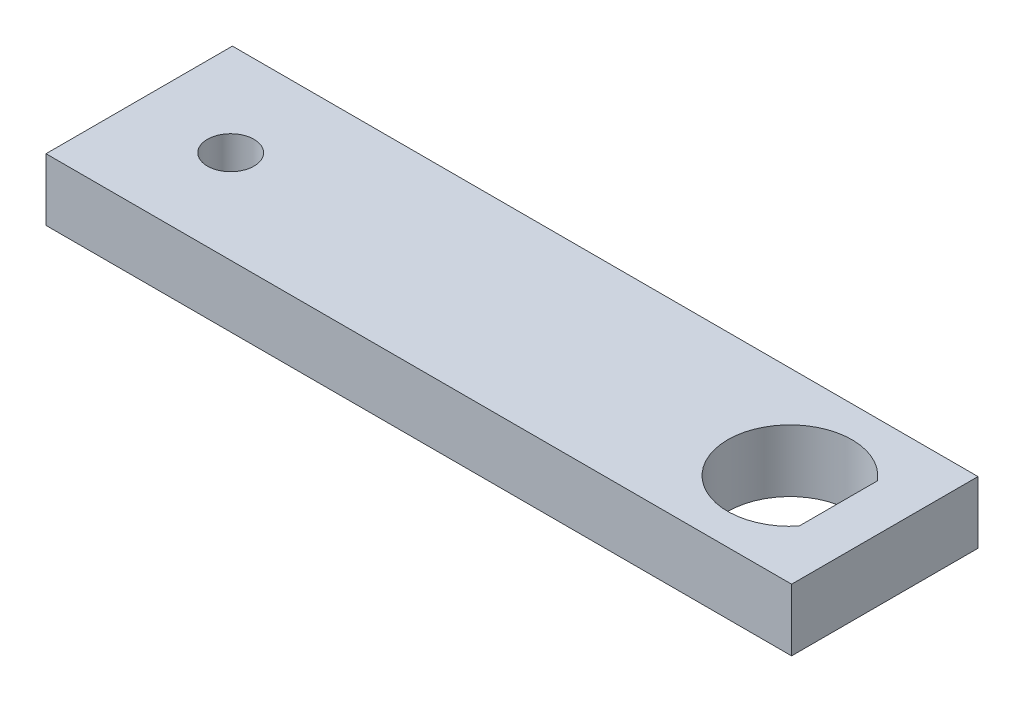
from build123d import *

# Parameters (mm, degrees)
BAR_OUTLINE_AND_HOLE_4_76_SKETCH_W = 76.2
BAR_OUTLINE_AND_HOLE_4_76_SKETCH_H = 19.05
BAR_OUTLINE_AND_HOLE_4_76_SKETCH_R = 2.38
LINK_BAR_6_35_THICK_DEPTH          = 6.35
D_HOLE_12_7_CUT_DEPTH              = 6.35


with BuildPart() as part:
    # Bar Outline and Hole Ø4.76 Sketch → Link Bar 6.35 Thick (new body)
    with BuildSketch(Plane(origin=(0, 0, 0), x_dir=(1, 0, 0), z_dir=(0, 1, 0))):
        Rectangle(BAR_OUTLINE_AND_HOLE_4_76_SKETCH_W, BAR_OUTLINE_AND_HOLE_4_76_SKETCH_H)
        with Locations(Location((-28.75, 0, 0), (0, 0, 270))):
            Circle(BAR_OUTLINE_AND_HOLE_4_76_SKETCH_R, mode=Mode.SUBTRACT)
    extrude(amount=LINK_BAR_6_35_THICK_DEPTH)

    # D-Hole Ø12.7 Sketch → D-Hole Ø12.7 Cut (cut)
    with BuildSketch(Plane(origin=(0, 6.35, 0), x_dir=(1, 0, 0), z_dir=(0, 1, 0))):
        with BuildLine():
            Line((33.34, -3.989849621), (33.34, 3.989849621))
            ThreePointArc((33.34, 3.989849621), (22.05, 0), (33.34, -3.989849621))
        make_face()
    extrude(amount=-D_HOLE_12_7_CUT_DEPTH, mode=Mode.SUBTRACT)


solid = part.part
